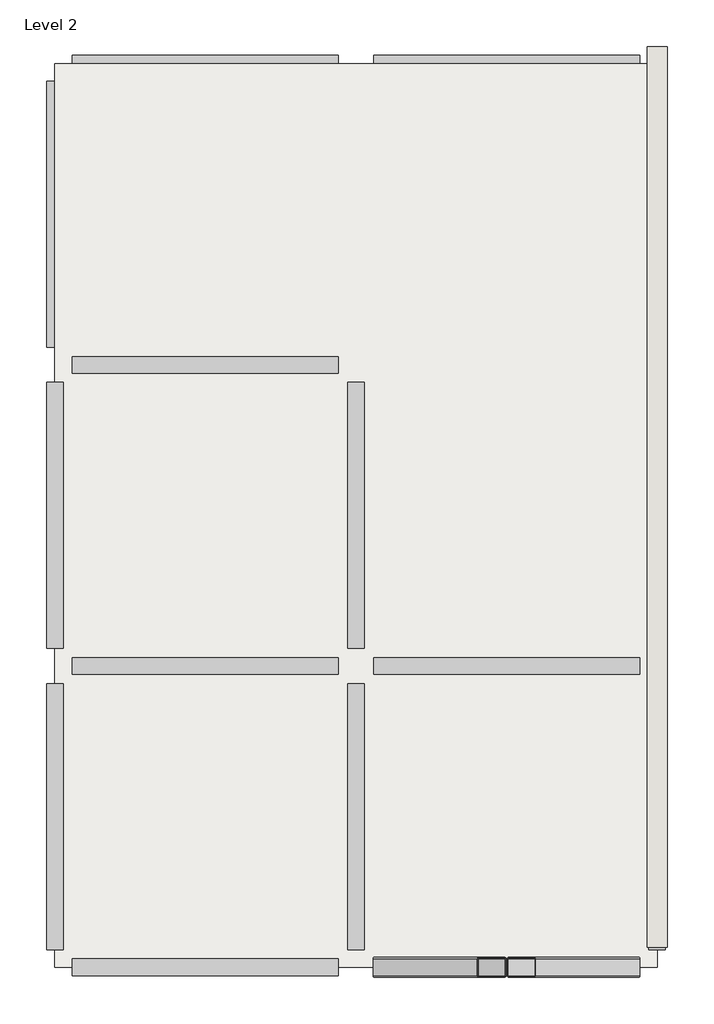
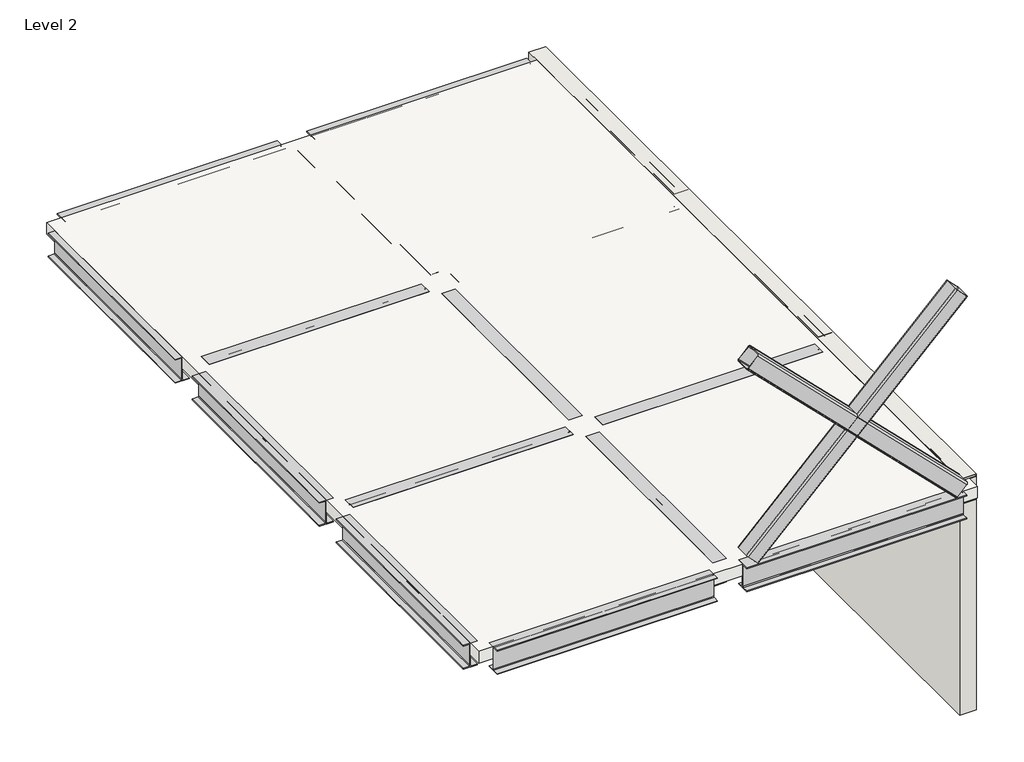
# One storey: 17 beams, 2 members, 1 slab, 1 wall.
"""IFC4 building model written with IfcOpenShell, lengths in millimetres."""

from ifc_helpers import new_model, si_unit, frame, origin, place, context, project, spatial, polyline, outline, extrude, faceted_brep, transform, mapped, element, save
from components import ub_universal_beams_ub305x165x40_60ab2ee1, m_hss_square_hss203_2x203_2x9_5_07d005dd

model = new_model("IFC4")

# Units and contexts
model_context = context("Model", 3, world=origin())
ifc_project = project(units=[si_unit("LENGTHUNIT", "METRE", prefix="MILLI")], contexts=[model_context])

# Site, building, storey
site = spatial("IfcSite", under=ifc_project)
building = spatial("IfcBuilding", under=site)
storey = spatial("IfcBuildingStorey", under=building, Name="Level 2", Elevation=3000.0)

# Beams
placement = place(None, origin())
ub_universal_beams_ub305x165x40_shape = ub_universal_beams_ub305x165x40_60ab2ee1(model_context)
element("IfcBeam", 1, ObjectType="UB-Universal Beams : UB305x165x40", at=placement, inside=storey, context=model_context, shape_type="MappedRepresentation", body=[
    mapped(ub_universal_beams_ub305x165x40_shape, transform((18435.1404262, -6314.7314166, 2848.3), x_axis=(-1.0, 0.0, 0.0), y_axis=(0.0, -1.0, 0.0), z_axis=(0.0, 0.0, 1.0))),
])
element("IfcBeam", 2, ObjectType="UB-Universal Beams : UB305x165x40", at=placement, inside=storey, context=model_context, shape_type="MappedRepresentation", body=[
    mapped(ub_universal_beams_ub305x165x40_shape, transform((15435.1404262, -6314.7314166, 2848.3), x_axis=(-1.0, 0.0, 0.0), y_axis=(0.0, -1.0, 0.0), z_axis=(0.0, 0.0, 1.0))),
])
element("IfcBeam", 3, ObjectType="UB-Universal Beams : UB305x165x40", at=placement, inside=storey, context=model_context, shape_type="MappedRepresentation", body=[
    mapped(ub_universal_beams_ub305x165x40_shape, transform((13935.1404262, -4814.7314166, 2848.3), x_axis=(0.0, 1.0, 0.0), y_axis=(-1.0, 0.0, 0.0), z_axis=(0.0, 0.0, 1.0))),
])
element("IfcBeam", 4, ObjectType="UB-Universal Beams : UB305x165x40", at=placement, inside=storey, context=model_context, shape_type="MappedRepresentation", body=[
    mapped(ub_universal_beams_ub305x165x40_shape, transform((13935.1404262, -1814.7314166, 2848.3), x_axis=(0.0, 1.0, 0.0), y_axis=(-1.0, 0.0, 0.0), z_axis=(0.0, 0.0, 1.0))),
])
element("IfcBeam", 5, ObjectType="UB-Universal Beams : UB305x165x40", at=placement, inside=storey, context=model_context, shape_type="MappedRepresentation", body=[
    mapped(ub_universal_beams_ub305x165x40_shape, transform((13935.1404262, 1185.2685834, 2848.3), x_axis=(0.0, 1.0, 0.0), y_axis=(-1.0, 0.0, 0.0), z_axis=(0.0, 0.0, 1.0))),
])
element("IfcBeam", 6, ObjectType="UB-Universal Beams : UB305x165x40", at=placement, inside=storey, context=model_context, shape_type="MappedRepresentation", body=[
    mapped(ub_universal_beams_ub305x165x40_shape, transform((18435.1404262, -3314.7314166, 2848.3), x_axis=(-1.0, 0.0, 0.0), y_axis=(0.0, -1.0, 0.0), z_axis=(0.0, 0.0, 1.0))),
])
element("IfcBeam", 7, ObjectType="UB-Universal Beams : UB305x165x40", at=placement, inside=storey, context=model_context, shape_type="MappedRepresentation", body=[
    mapped(ub_universal_beams_ub305x165x40_shape, transform((15435.1404262, -3314.7314166, 2848.3), x_axis=(-1.0, 0.0, 0.0), y_axis=(0.0, -1.0, 0.0), z_axis=(0.0, 0.0, 1.0))),
])
element("IfcBeam", 8, ObjectType="UB-Universal Beams : UB305x165x40", at=placement, inside=storey, context=model_context, shape_type="MappedRepresentation", body=[
    mapped(ub_universal_beams_ub305x165x40_shape, transform((18435.1404262, -314.7314166, 2848.3), x_axis=(-1.0, 0.0, 0.0), y_axis=(0.0, -1.0, 0.0), z_axis=(0.0, 0.0, 1.0))),
])
element("IfcBeam", 9, ObjectType="UB-Universal Beams : UB305x165x40", at=placement, inside=storey, context=model_context, shape_type="MappedRepresentation", body=[
    mapped(ub_universal_beams_ub305x165x40_shape, transform((15435.1404262, -314.7314166, 2848.3), x_axis=(-1.0, 0.0, 0.0), y_axis=(0.0, -1.0, 0.0), z_axis=(0.0, 0.0, 1.0))),
])
element("IfcBeam", 10, ObjectType="UB-Universal Beams : UB305x165x40", at=placement, inside=storey, context=model_context, shape_type="MappedRepresentation", body=[
    mapped(ub_universal_beams_ub305x165x40_shape, transform((18435.1404262, 2685.2685834, 2848.3), x_axis=(-1.0, 0.0, 0.0), y_axis=(0.0, -1.0, 0.0), z_axis=(0.0, 0.0, 1.0))),
])
element("IfcBeam", 11, ObjectType="UB-Universal Beams : UB305x165x40", at=placement, inside=storey, context=model_context, shape_type="MappedRepresentation", body=[
    mapped(ub_universal_beams_ub305x165x40_shape, transform((15435.1404262, 2685.2685834, 2848.3), x_axis=(-1.0, 0.0, 0.0), y_axis=(0.0, -1.0, 0.0), z_axis=(0.0, 0.0, 1.0))),
])
element("IfcBeam", 12, ObjectType="UB-Universal Beams : UB305x165x40", at=placement, inside=storey, context=model_context, shape_type="MappedRepresentation", body=[
    mapped(ub_universal_beams_ub305x165x40_shape, transform((16935.1404262, -4814.7314166, 2848.3), x_axis=(0.0, 1.0, 0.0), y_axis=(-1.0, 0.0, 0.0), z_axis=(0.0, 0.0, 1.0))),
])
element("IfcBeam", 13, ObjectType="UB-Universal Beams : UB305x165x40", at=placement, inside=storey, context=model_context, shape_type="MappedRepresentation", body=[
    mapped(ub_universal_beams_ub305x165x40_shape, transform((16935.1404262, -1814.7314166, 2848.3), x_axis=(0.0, 1.0, 0.0), y_axis=(-1.0, 0.0, 0.0), z_axis=(0.0, 0.0, 1.0))),
])
element("IfcBeam", 14, ObjectType="UB-Universal Beams : UB305x165x40", at=placement, inside=storey, context=model_context, shape_type="MappedRepresentation", body=[
    mapped(ub_universal_beams_ub305x165x40_shape, transform((16935.1404262, 1185.2685834, 2848.3), x_axis=(0.0, 1.0, 0.0), y_axis=(-1.0, 0.0, 0.0), z_axis=(0.0, 0.0, 1.0))),
])
element("IfcBeam", 15, ObjectType="UB-Universal Beams : UB305x165x40", at=placement, inside=storey, context=model_context, shape_type="MappedRepresentation", body=[
    mapped(ub_universal_beams_ub305x165x40_shape, transform((19935.1404262, -1814.7314166, 2848.3), x_axis=(0.0, 1.0, 0.0), y_axis=(-1.0, 0.0, 0.0), z_axis=(0.0, 0.0, 1.0))),
])
element("IfcBeam", 16, ObjectType="UB-Universal Beams : UB305x165x40", at=placement, inside=storey, context=model_context, shape_type="MappedRepresentation", body=[
    mapped(ub_universal_beams_ub305x165x40_shape, transform((19935.1404262, 1185.2685834, 2848.3), x_axis=(0.0, 1.0, 0.0), y_axis=(-1.0, 0.0, 0.0), z_axis=(0.0, 0.0, 1.0))),
])
element("IfcBeam", 17, ObjectType="UB-Universal Beams : beam", at=placement, inside=storey, context=model_context, shape_type="MappedRepresentation", body=[
    mapped(ub_universal_beams_ub305x165x40_shape, transform((19935.1404262, -4814.7314166, 2848.3), x_axis=(0.0, 1.0, 0.0), y_axis=(-1.0, 0.0, 0.0), z_axis=(0.0, 0.0, 1.0))),
])

# Members
m_hss_square_hss203_2x203_2x9_5_shape = m_hss_square_hss203_2x203_2x9_5_07d005dd(model_context)
element("IfcMember", 18, ObjectType="M_HSS Square : HSS203.2X203.2X9.5", at=placement, inside=storey, context=model_context, shape_type="MappedRepresentation", body=[
    mapped(m_hss_square_hss203_2x203_2x9_5_shape, transform((18435.1404262, -6314.7314166, 4348.3), x_axis=(-0.7071067811865478, 0.0, 0.7071067811865476), y_axis=(0.0, -1.0000000000000002, 0.0), z_axis=(0.7071067811865476, 0.0, 0.7071067811865478))),
])
element("IfcMember", 19, ObjectType="M_HSS Square : HSS203.2X203.2X9.5", at=placement, inside=storey, context=model_context, shape_type="MappedRepresentation", body=[
    mapped(m_hss_square_hss203_2x203_2x9_5_shape, transform((18435.1404262, -6314.7314166, 4348.3), x_axis=(-0.7071067811865478, 0.0, -0.7071067811865475), y_axis=(0.0, -1.0000000000000002, 0.0), z_axis=(-0.7071067811865475, 0.0, 0.7071067811865478))),
])

# Slab
element("IfcSlab", 20, ObjectType="150mm Foundation Slab", at=placement, inside=storey, context=model_context, shape_type="SweptSolid", body=[
    extrude(outline(polyline([(13935.1404262, -6314.7314166), (13935.1404262, 2685.2685834), (19935.1404262, 2685.2685834), (19935.1404262, -6314.7314166), (13935.1404262, -6314.7314166)])), frame((0.0, 0.0, 2850.0), z_axis=(0.0, 0.0, 1.0), x_axis=(1.0, 0.0, 0.0)), (0.0, 0.0, 1.0), 150.0),
])

# Wall
element("IfcWall", 21, ObjectType="Generic - 200mm", at=placement, inside=storey, context=model_context, shape_type="Brep", body=[
    faceted_brep([(19835.1404262, 2855.9792615, 0.0), (19835.1404262, 2655.9792615, 0.0), (19835.1404262, -6114.7314166, 0.0), (19835.1404262, -6114.7314166, 3000.0), (19835.1404262, 2655.9792615, 3000.0), (19835.1404262, 2855.9792615, 3000.0), (20035.1404262, 2855.9792615, 0.0), (20035.1404262, 2855.9792615, 3000.0), (20035.1404262, 2655.9792615, 3000.0), (20035.1404262, -6114.7314166, 3000.0), (20035.1404262, -6114.7314166, 0.0)], [[[0, 1, 2, 3, 4, 5]], [[6, 7, 8, 9, 10]], [[2, 1, 0, 6, 10]], [[5, 4, 3, 9, 8, 7]], [[3, 2, 10, 9]], [[0, 5, 7, 6]]]),
])

save(model, "model.ifc")

# Revit data of these elements
# Type "UB-Universal Beams : UB305x165x40"
#   Section Name Key = "UB305X165X40"
#   Width = 16.5 cm
#   Web Thickness = 0.6 cm
#   Web Fillet = 0.89 cm
#   Warping Constant = 164000.0 cm⁶
#   Torsional Moment of Inertia = 14.70 cm⁴
#   Section Area = 51.3 cm²
#   Plastic Modulus weak axis = 142.0 cm³
#   Plastic Modulus strong axis = 623.0 cm³
#   Nominal Weight = 40.2999 kgf/m
#   Moment of Inertia weak axis = 764.00 cm⁴
#   Moment of Inertia strong axis = 8503.00 cm⁴
#   Height = 30.34 cm
#   Flange Thickness = 1.02 cm
#   Elastic Modulus weak axis = 92.6 cm³
#   Elastic Modulus strong axis = 560.0 cm³
#   Centroid Vertical = 15.17 cm
#   Centroid Horizontal = 8.25 cm
#   Bolt Spacing = 9.0 cm
#   Length [instance default] = 1.5 m
#   Structural Material [instance default] = Metal - Steel 43-275
#   Type Comments = ""
#   Assembly Code = ""
# Type "UB-Universal Beams : beam"
#   Section Name Key = "UB305X165X40"
#   Width = 16.5 cm
#   Web Thickness = 0.6 cm
#   Web Fillet = 0.89 cm
#   Warping Constant = 164000.0 cm⁶
#   Torsional Moment of Inertia = 14.70 cm⁴
#   Section Area = 51.3 cm²
#   Plastic Modulus weak axis = 142.0 cm³
#   Plastic Modulus strong axis = 623.0 cm³
#   Nominal Weight = 40.2999 kgf/m
#   Moment of Inertia weak axis = 764.00 cm⁴
#   Moment of Inertia strong axis = 8503.00 cm⁴
#   Height = 30.34 cm
#   Flange Thickness = 1.02 cm
#   Elastic Modulus weak axis = 92.6 cm³
#   Elastic Modulus strong axis = 560.0 cm³
#   Centroid Vertical = 15.17 cm
#   Centroid Horizontal = 8.25 cm
#   Bolt Spacing = 9.0 cm
#   Length [instance default] = 1.5 m
#   Structural Material [instance default] = Metal - Steel 43-275
#   Type Comments = ""
#   Assembly Code = ""
# Type "M_HSS Square : HSS203.2X203.2X9.5"
#   Section Name Key = "HSS 8X8X3/8"
#   Width = 20.3 cm
#   Wall Nominal Thickness = 0.953 cm
#   Wall Design Thickness = 0.886 cm
#   Torsional Moment of Inertia = 6660.00 cm⁴
#   Torsional Modulus = 10930171.7 cm³
#   Section Area = 67.1 cm²
#   Plastic Modulus weak axis = 482.0 cm³
#   Plastic Modulus strong axis = 482.0 cm³
#   Outer Fillet = 1.906 cm
#   Nominal Weight = 55.9998 kgf/m
#   Moment of Inertia weak axis = 4160.00 cm⁴
#   Moment of Inertia strong axis = 4160.00 cm⁴
#   Length [instance default] = 1.524 m
#   Inner Fillet = 0.953 cm
#   Height = 20.3 cm
#   Elastic Modulus weak axis = 408.0 cm³
#   Elastic Modulus strong axis = 408.0 cm³
#   Centroid Vertical = 10.15 cm
#   Centroid Horizontal = 10.15 cm
#   Structural Material [instance default] = Steel, 45-345
# Type "150mm Foundation Slab"
#   Layers, outside or top first: 0.15 m "Concrete, Cast-in-Place gray" (function 1)
# Type "Generic - 200mm"
#   Layers, outside or top first: 0.2 m no material (function 1)
# Elements 1, 2, 3, 4, 5, 6, 7, 8, 9, 10, 11, 12, 13, 14, 15, 16 (IfcBeam, "UB-Universal Beams : UB305x165x40")
#   Structural Material = Metal - Steel 43-275
#   Phase Created = New Construction
#   Materials on its faces: "Metal - Steel 43-275"
# Element 17 (IfcBeam, "UB-Universal Beams : beam")
#   Structural Material = Metal - Steel 43-275
#   Phase Created = New Construction
#   Materials on its faces: "Metal - Steel 43-275"
# Elements 18, 19 (IfcMember, "M_HSS Square : HSS203.2X203.2X9.5")
#   Comments = ""
#   Structural Material = Metal - Steel 43-275
#   Phase Created = New Construction
#   Materials on its faces: "Metal - Steel 43-275"
# Element 20 (IfcSlab, "150mm Foundation Slab")
#   built-in parameter 1001955 = 3.14159 (stored number, unit not read)
#   Height Offset From Level = 0 m
#   built-in parameter 1001954 = 1
#   Phase Created = New Construction
#   Materials on its faces: "Concrete, Cast-in-Place gray"
# Element 21 (IfcWall, "Generic - 200mm")
#   Comments = ""
#   built-in parameter 1001111 = -3 m
#   Top Offset = 0 m
#   Base Offset = -3 m
#   wall height = 3 m
#   Phase Created = New Construction
#   Base Constraint = Level 2
#   Top Constraint = Level 2
#   Materials on its faces: "Default Wall"
# Materials
#   "Metal - Steel 43-275": class "Metal", colour RGB 247 247 247, transparency 0, Cost = 0
#   "Steel, 45-345": class "Metal", colour RGB 247 247 247, transparency 0, Description = "Steel 345 MPa", Cost = 0
#   "Concrete, Cast-in-Place gray": class "Concrete", colour RGB 192 192 192, transparency 0, Description = "Cast-in-place concrete", Cost = 0
#   "Default Wall": colour RGB 128 128 128, transparency 0, Cost = 0
